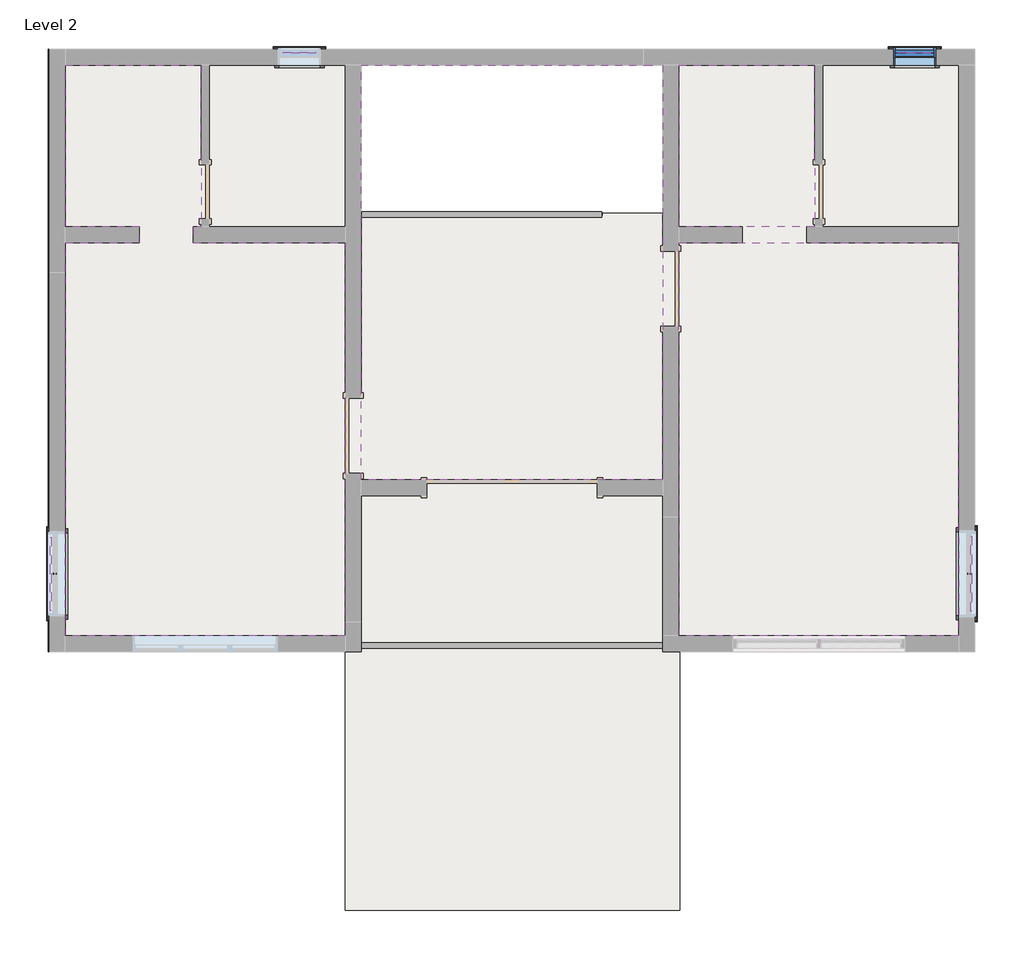
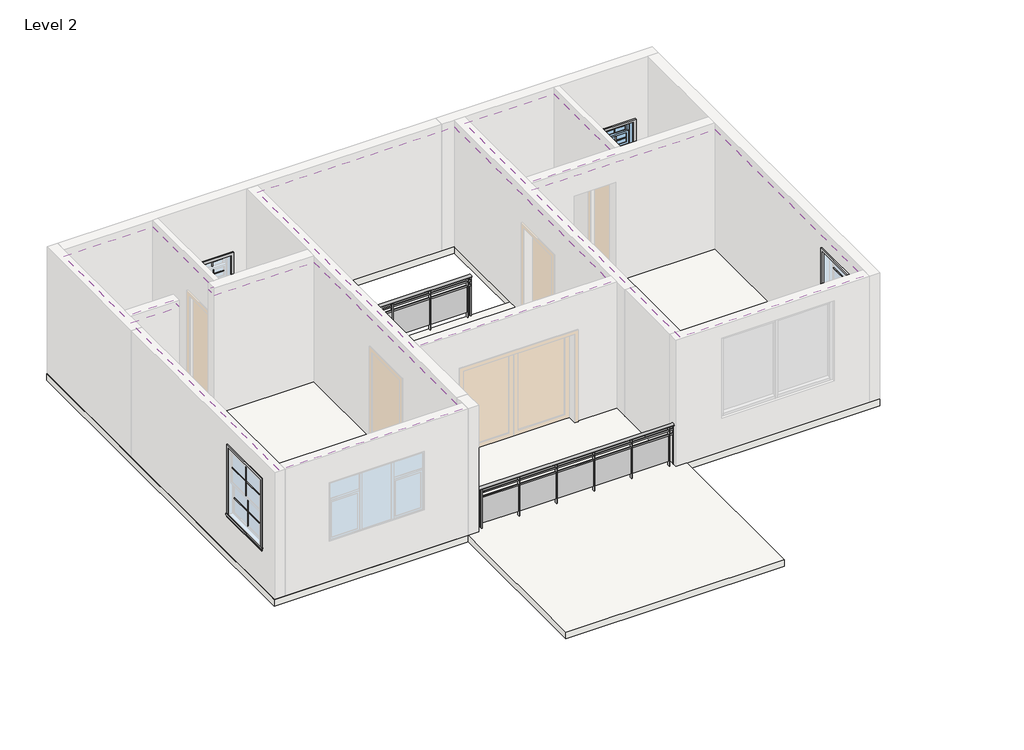
# One storey, part 2 of 2: 16 proxies, 4 coverings, 2 railings, 1 slab, 1 window.
"""IFC4 building model written with IfcOpenShell, lengths in millimetres."""

from ifc_helpers import new_model, si_unit, point, frame, origin, place, context, project, spatial, polyline, ellipse_curve, trimmed, outline, extrude, transform, mapped, element, save
from ifc_brep_helpers import plane_surface, extruded_surface, advanced_brep
from components import muntin_pattern_2x2_muntin_pattern_2x2_872d1288, muntin_pattern_2x2_muntin_pattern_2x2_cfeb24ad, muntin_pattern_2x2_muntin_pattern_2x2_afeb4eca, trim_window_exterior_flat_with_sill_c3105ee7, trim_window_exterior_flat_with_sill_858dc10d, trim_window_exterior_flat_with_sill_92b9b949, trim_window_interior_flat_picture_frame_d5efd988, trim_window_interior_flat_picture_frame_3927330c, trim_window_interior_flat_picture_frame_3bb882cf, window_double_hung_2_x2_15b2d83c

model = new_model("IFC4")

# Units and contexts
model_context = context("Model", 3, world=origin())
ifc_project = project(units=[si_unit("LENGTHUNIT", "METRE", prefix="MILLI")], contexts=[model_context])

# Site, building, storey
site = spatial("IfcSite", under=ifc_project)
building = spatial("IfcBuilding", under=site)
storey = spatial("IfcBuildingStorey", under=building, Name="Level 2", Elevation=3048.0)

# Proxies
placement = place(None, origin())
muntin_pattern_2x2_muntin_pattern_2x2_shape = muntin_pattern_2x2_muntin_pattern_2x2_872d1288(model_context)
element("IfcBuildingElementProxy", 1, Name="Muntin Pattern_2x2 : Muntin Pattern_2x2", ObjectType="Muntin Pattern_2x2 : Muntin Pattern_2x2", at=placement, inside=storey, context=model_context, shape_type="MappedRepresentation", body=[
    mapped(muntin_pattern_2x2_muntin_pattern_2x2_shape, transform((-19390.8072207, 4603.0962903, 4746.625), x_axis=(0.0, 1.0, 0.0), y_axis=(-1.0, 0.0, 0.0), z_axis=(0.0, 0.0, 1.0))),
])
element("IfcBuildingElementProxy", 2, Name="Muntin Pattern_2x2 : Muntin Pattern_2x2", ObjectType="Muntin Pattern_2x2 : Muntin Pattern_2x2", at=placement, inside=storey, context=model_context, shape_type="MappedRepresentation", body=[
    mapped(muntin_pattern_2x2_muntin_pattern_2x2_shape, transform((-19346.3572207, 4603.0962903, 4038.6), x_axis=(0.0, 1.0, 0.0), y_axis=(-1.0, 0.0, 0.0), z_axis=(0.0, 0.0, 1.0))),
])
muntin_pattern_2x2_muntin_pattern_2x2_2_shape = muntin_pattern_2x2_muntin_pattern_2x2_cfeb24ad(model_context)
element("IfcBuildingElementProxy", 3, Name="Muntin Pattern_2x2 : Muntin Pattern_2x2", ObjectType="Muntin Pattern_2x2 : Muntin Pattern_2x2", at=placement, inside=storey, context=model_context, shape_type="MappedRepresentation", body=[
    mapped(muntin_pattern_2x2_muntin_pattern_2x2_2_shape, transform((-15881.0556236, 11998.6707578, 4289.425), x_axis=(1.0, 0.0, 0.0), y_axis=(0.0, 1.0, 0.0), z_axis=(0.0, 0.0, 1.0))),
])
element("IfcBuildingElementProxy", 4, Name="Muntin Pattern_2x2 : Muntin Pattern_2x2", ObjectType="Muntin Pattern_2x2 : Muntin Pattern_2x2", at=placement, inside=storey, context=model_context, shape_type="MappedRepresentation", body=[
    mapped(muntin_pattern_2x2_muntin_pattern_2x2_2_shape, transform((-15881.0556236, 11954.2207578, 4038.6), x_axis=(1.0, 0.0, 0.0), y_axis=(0.0, 1.0, 0.0), z_axis=(0.0, 0.0, 1.0))),
])
element("IfcBuildingElementProxy", 5, Name="Muntin Pattern_2x2 : Muntin Pattern_2x2", ObjectType="Muntin Pattern_2x2 : Muntin Pattern_2x2", at=placement, inside=storey, context=model_context, shape_type="MappedRepresentation", body=[
    mapped(muntin_pattern_2x2_muntin_pattern_2x2_2_shape, transform((-7166.2817031, 11998.6707578, 4289.425), x_axis=(1.0, 0.0, 0.0), y_axis=(0.0, 1.0, 0.0), z_axis=(0.0, 0.0, 1.0))),
])
element("IfcBuildingElementProxy", 6, Name="Muntin Pattern_2x2 : Muntin Pattern_2x2", ObjectType="Muntin Pattern_2x2 : Muntin Pattern_2x2", at=placement, inside=storey, context=model_context, shape_type="MappedRepresentation", body=[
    mapped(muntin_pattern_2x2_muntin_pattern_2x2_2_shape, transform((-7166.2817031, 11954.2207578, 4038.6), x_axis=(1.0, 0.0, 0.0), y_axis=(0.0, 1.0, 0.0), z_axis=(0.0, 0.0, 1.0))),
])
muntin_pattern_2x2_muntin_pattern_2x2_3_shape = muntin_pattern_2x2_muntin_pattern_2x2_afeb4eca(model_context)
element("IfcBuildingElementProxy", 7, Name="Muntin Pattern_2x2 : Muntin Pattern_2x2", ObjectType="Muntin Pattern_2x2 : Muntin Pattern_2x2", at=placement, inside=storey, context=model_context, shape_type="MappedRepresentation", body=[
    mapped(muntin_pattern_2x2_muntin_pattern_2x2_3_shape, transform((-6350.3067031, 4603.0962903, 4746.625), x_axis=(0.0, -1.0, 0.0), y_axis=(1.0, 0.0, 0.0), z_axis=(0.0, 0.0, 1.0))),
])
element("IfcBuildingElementProxy", 8, Name="Muntin Pattern_2x2 : Muntin Pattern_2x2", ObjectType="Muntin Pattern_2x2 : Muntin Pattern_2x2", at=placement, inside=storey, context=model_context, shape_type="MappedRepresentation", body=[
    mapped(muntin_pattern_2x2_muntin_pattern_2x2_3_shape, transform((-6394.7567031, 4603.0962903, 4038.6), x_axis=(0.0, -1.0, 0.0), y_axis=(1.0, 0.0, 0.0), z_axis=(0.0, 0.0, 1.0))),
])
trim_window_exterior_flat_with_sill_shape = trim_window_exterior_flat_with_sill_c3105ee7(model_context)
element("IfcBuildingElementProxy", 9, Name="Trim-Window-Exterior-Flat : with Sill", ObjectType="Trim-Window-Exterior-Flat : with Sill", at=placement, inside=storey, context=model_context, shape_type="MappedRepresentation", body=[
    mapped(trim_window_exterior_flat_with_sill_shape, transform((-19425.7322207, 4603.0962903, 5486.4), x_axis=(0.0, -1.0, 0.0), y_axis=(0.0, 0.0, 1.0), z_axis=(-1.0, 0.0, 0.0))),
])
trim_window_exterior_flat_with_sill_2_shape = trim_window_exterior_flat_with_sill_858dc10d(model_context)
element("IfcBuildingElementProxy", 10, Name="Trim-Window-Exterior-Flat : with Sill", ObjectType="Trim-Window-Exterior-Flat : with Sill", at=placement, inside=storey, context=model_context, shape_type="MappedRepresentation", body=[
    mapped(trim_window_exterior_flat_with_sill_2_shape, transform((-15881.0556236, 12033.5957578, 4572.0), x_axis=(-1.0, 0.0, 0.0), y_axis=(0.0, 0.0, 1.0), z_axis=(0.0, 1.0, 0.0))),
])
element("IfcBuildingElementProxy", 11, Name="Trim-Window-Exterior-Flat : with Sill", ObjectType="Trim-Window-Exterior-Flat : with Sill", at=placement, inside=storey, context=model_context, shape_type="MappedRepresentation", body=[
    mapped(trim_window_exterior_flat_with_sill_2_shape, transform((-7166.2817031, 12033.5957578, 4572.0), x_axis=(-1.0, 0.0, 0.0), y_axis=(0.0, 0.0, 1.0), z_axis=(0.0, 1.0, 0.0))),
])
trim_window_exterior_flat_with_sill_3_shape = trim_window_exterior_flat_with_sill_92b9b949(model_context)
element("IfcBuildingElementProxy", 12, Name="Trim-Window-Exterior-Flat : with Sill", ObjectType="Trim-Window-Exterior-Flat : with Sill", at=placement, inside=storey, context=model_context, shape_type="MappedRepresentation", body=[
    mapped(trim_window_exterior_flat_with_sill_3_shape, transform((-6315.3817031, 4603.0962903, 5486.4), x_axis=(0.0, 1.0, 0.0), y_axis=(0.0, 0.0, 1.0), z_axis=(1.0, 0.0, 0.0))),
])
trim_window_interior_flat_picture_frame_shape = trim_window_interior_flat_picture_frame_d5efd988(model_context)
element("IfcBuildingElementProxy", 13, Name="Trim-Window-Interior-Flat : Picture Frame", ObjectType="Trim-Window-Interior-Flat : Picture Frame", at=placement, inside=storey, context=model_context, shape_type="MappedRepresentation", body=[
    mapped(trim_window_interior_flat_picture_frame_shape, transform((-19197.1322207, 4603.0962903, 5486.4), x_axis=(0.0, 1.0, 0.0), y_axis=(0.0, 0.0, 1.0), z_axis=(1.0, 0.0, 0.0))),
])
trim_window_interior_flat_picture_frame_2_shape = trim_window_interior_flat_picture_frame_3927330c(model_context)
element("IfcBuildingElementProxy", 14, Name="Trim-Window-Interior-Flat : Picture Frame", ObjectType="Trim-Window-Interior-Flat : Picture Frame", at=placement, inside=storey, context=model_context, shape_type="MappedRepresentation", body=[
    mapped(trim_window_interior_flat_picture_frame_2_shape, transform((-15881.0556236, 11804.9957578, 4572.0), x_axis=(1.0, 0.0, 0.0), y_axis=(0.0, 0.0, 1.0), z_axis=(0.0, -1.0, 0.0))),
])
element("IfcBuildingElementProxy", 15, Name="Trim-Window-Interior-Flat : Picture Frame", ObjectType="Trim-Window-Interior-Flat : Picture Frame", at=placement, inside=storey, context=model_context, shape_type="MappedRepresentation", body=[
    mapped(trim_window_interior_flat_picture_frame_2_shape, transform((-7166.2817031, 11804.9957578, 4572.0), x_axis=(1.0, 0.0, 0.0), y_axis=(0.0, 0.0, 1.0), z_axis=(0.0, -1.0, 0.0))),
])
trim_window_interior_flat_picture_frame_3_shape = trim_window_interior_flat_picture_frame_3bb882cf(model_context)
element("IfcBuildingElementProxy", 16, Name="Trim-Window-Interior-Flat : Picture Frame", ObjectType="Trim-Window-Interior-Flat : Picture Frame", at=placement, inside=storey, context=model_context, shape_type="MappedRepresentation", body=[
    mapped(trim_window_interior_flat_picture_frame_3_shape, transform((-6543.9817031, 4603.0962903, 5486.4), x_axis=(0.0, -1.0, 0.0), y_axis=(0.0, 0.0, 1.0), z_axis=(-1.0, 0.0, 0.0))),
])

# Coverings
element("IfcCovering", 17, ObjectType="2' x 4' ACT System", at=placement, inside=storey, context=model_context, shape_type="SweptSolid", body=[
    extrude(outline(polyline([(-6543.9817031, 9289.635577), (-6543.9817031, 3726.7962903), (-10507.7583002, 3726.7962903), (-10507.7583002, 5401.1206207), (-10509.1026022, 5401.1206207), (-10509.1026022, 9289.635577), (-6543.9817031, 9289.635577)])), frame((0.0, 0.0, 5791.2), z_axis=(0.0, 0.0, 1.0), x_axis=(1.0, 0.0, 0.0)), (0.0, 0.0, 1.0), 57.15),
])
element("IfcCovering", 18, ObjectType="2' x 4' ACT System", at=placement, inside=storey, context=model_context, shape_type="SweptSolid", body=[
    extrude(outline(polyline([(-10509.1026022, 9518.235577), (-10509.1026022, 11804.9957578), (-8581.223198, 11804.9957578), (-8581.223198, 9518.235577), (-10509.1026022, 9518.235577)])), frame((0.0, 0.0, 5791.2), z_axis=(0.0, 0.0, 1.0), x_axis=(1.0, 0.0, 0.0)), (0.0, 0.0, 1.0), 57.15),
])
element("IfcCovering", 19, ObjectType="2' x 4' ACT System", at=placement, inside=storey, context=model_context, shape_type="SweptSolid", body=[
    extrude(outline(polyline([(-15004.7556236, 5935.1163046), (-15004.7556236, 11804.9957578), (-11009.5531945, 11804.9957578), (-10737.7026022, 11804.9957578), (-10737.7026022, 5935.1163046), (-15004.7556236, 5935.1163046)])), frame((0.0, 0.0, 5791.2), z_axis=(0.0, 0.0, 1.0), x_axis=(1.0, 0.0, 0.0)), (0.0, 0.0, 1.0), 57.15),
])
element("IfcCovering", 20, ObjectType="2' x 4' ACT System", at=placement, inside=storey, context=model_context, shape_type="SweptSolid", body=[
    extrude(outline(polyline([(-19197.1322207, 9290.2207935), (-18149.1852461, 9290.2207935), (-18149.1852461, 9518.8207935), (-19197.1322207, 9518.8207935), (-19197.1322207, 11804.9957578), (-17272.3740665, 11804.9957578), (-17272.3740665, 9518.8207935), (-17388.0183685, 9518.8207935), (-17388.0183685, 9290.2207935), (-15233.3556236, 9290.2207935), (-15233.3556236, 3726.7962903), (-19197.1322207, 3726.7962903), (-19197.1322207, 9290.2207935)])), frame((0.0, 0.0, 5791.2), z_axis=(0.0, 0.0, 1.0), x_axis=(1.0, 0.0, 0.0)), (0.0, 0.0, 1.0), 57.15),
])

# Railings
element("IfcRailing", 21, ObjectType="Glass Panel - Bottom Fill", at=placement, inside=storey, context=model_context, shape_type="SolidModel", body=[
    advanced_brep(
    [(-15004.5982861, 9732.8204925, 3962.4), (-15004.5982861, 9656.6204925, 3962.4), (-11600.9982861, 9732.8204925, 3962.4), (-11600.9982861, 9656.6204925, 3962.4)],
    [
        (0, 1, ellipse_curve(frame((-15004.5982861, 9694.7204925, 3962.4), z_axis=(-1.0, 0.0, 0.0), x_axis=(0.0, -1.0, 0.0)), 38.1, 28.575)),
        (1, 0, ellipse_curve(frame((-15004.5982861, 9694.7204925, 3962.4), z_axis=(-1.0, 0.0, 0.0), x_axis=(0.0, -1.0, 0.0)), 38.1, 28.575)),
        (2, 3, ellipse_curve(frame((-11600.9982861, 9694.7204925, 3962.4), z_axis=(1.0, 0.0, 0.0), x_axis=(0.0, -1.0, 0.0)), 38.1, 28.575)),
        (3, 2, ellipse_curve(frame((-11600.9982861, 9694.7204925, 3962.4), z_axis=(1.0, 0.0, 0.0), x_axis=(0.0, -1.0, 0.0)), 38.1, 28.575)),
        (0, 2),
        (3, 1),
    ],
    [
        plane_surface(frame((-15004.5982861, 9694.7204925, 3962.4), z_axis=(-1.0, 0.0, 0.0), x_axis=(0.0, 1.0, 0.0))),
        plane_surface(frame((-11600.9982861, 9694.7204925, 3962.4), z_axis=(1.0, 0.0, 0.0), x_axis=(0.0, 1.0, 0.0))),
        extruded_surface(trimmed(ellipse_curve(frame((-11600.9982861, 9694.7204925, 3962.4), z_axis=(-1.0, 0.0, 0.0), x_axis=(0.0, -1.0, 0.0)), 38.1, 28.575), [point((-11600.9982861, 9732.8204925, 3962.4))], [point((-11600.9982861, 9656.6204925, 3962.4))], True, "CARTESIAN"), (-3403.5999999999985, 0.0, 0.0), 3403.5999999999985),
        extruded_surface(trimmed(ellipse_curve(frame((-11600.9982861, 9694.7204925, 3962.4), z_axis=(-1.0, 0.0, 0.0), x_axis=(0.0, -1.0, 0.0)), 38.1, 28.575), [point((-11600.9982861, 9656.6204925, 3962.4))], [point((-11600.9982861, 9732.8204925, 3962.4))], True, "CARTESIAN"), (-3403.5999999999985, 0.0, 0.0), 3403.5999999999985),
    ],
    [
        (0, [[1, 2]]),
        (1, [[3, 4]]),
        (2, [[-1, 5, -4, 6]]),
        (3, [[-2, -6, -3, -5]]),
    ],
),
    extrude(outline(polyline([(-15004.5982861, 9682.0204925), (-15004.5982861, 9707.4204925), (-11600.9982861, 9707.4204925), (-11600.9982861, 9682.0204925), (-15004.5982861, 9682.0204925)])), frame((0.0, 0.0, 3848.1), z_axis=(0.0, 0.0, 1.0), x_axis=(1.0, 0.0, 0.0)), (0.0, 0.0, 1.0), 25.4),
    extrude(outline(polyline([(-15004.5982861, 9682.0204925), (-15004.5982861, 9707.4204925), (-11600.9982861, 9707.4204925), (-11600.9982861, 9682.0204925), (-15004.5982861, 9682.0204925)])), frame((0.0, 0.0, 3746.5), z_axis=(0.0, 0.0, 1.0), x_axis=(1.0, 0.0, 0.0)), (0.0, 0.0, 1.0), 25.4),
    extrude(outline(polyline([(-11683.5482861, 9669.3204925), (-11683.5482861, 9720.1204925), (-11670.8482861, 9720.1204925), (-11670.8482861, 9669.3204925), (-11683.5482861, 9669.3204925)])), frame((0.0, 0.0, 3048.0), z_axis=(0.0, 0.0, 1.0), x_axis=(1.0, 0.0, 0.0)), (0.0, 0.0, 1.0), 885.825),
    extrude(outline(polyline([(-12489.9982861, 9701.2556495), (-11677.1982861, 9701.2556495), (-11677.1982861, 9694.9056495), (-12489.9982861, 9694.9056495), (-12489.9982861, 9701.2556495)])), frame((0.0, 0.0, 3149.6), z_axis=(0.0, 0.0, 1.0), x_axis=(1.0, 0.0, 0.0)), (0.0, 0.0, 1.0), 596.9),
    extrude(outline(polyline([(-12496.3482861, 9669.3204925), (-12496.3482861, 9720.1204925), (-12483.6482861, 9720.1204925), (-12483.6482861, 9669.3204925), (-12496.3482861, 9669.3204925)])), frame((0.0, 0.0, 3048.0), z_axis=(0.0, 0.0, 1.0), x_axis=(1.0, 0.0, 0.0)), (0.0, 0.0, 1.0), 885.825),
    extrude(outline(polyline([(-13302.7982861, 9701.2556495), (-12489.9982861, 9701.2556495), (-12489.9982861, 9694.9056495), (-13302.7982861, 9694.9056495), (-13302.7982861, 9701.2556495)])), frame((0.0, 0.0, 3149.6), z_axis=(0.0, 0.0, 1.0), x_axis=(1.0, 0.0, 0.0)), (0.0, 0.0, 1.0), 596.9),
    extrude(outline(polyline([(-13309.1482861, 9669.3204925), (-13309.1482861, 9720.1204925), (-13296.4482861, 9720.1204925), (-13296.4482861, 9669.3204925), (-13309.1482861, 9669.3204925)])), frame((0.0, 0.0, 3048.0), z_axis=(0.0, 0.0, 1.0), x_axis=(1.0, 0.0, 0.0)), (0.0, 0.0, 1.0), 885.825),
    extrude(outline(polyline([(-14115.5982861, 9701.2556495), (-13302.7982861, 9701.2556495), (-13302.7982861, 9694.9056495), (-14115.5982861, 9694.9056495), (-14115.5982861, 9701.2556495)])), frame((0.0, 0.0, 3149.6), z_axis=(0.0, 0.0, 1.0), x_axis=(1.0, 0.0, 0.0)), (0.0, 0.0, 1.0), 596.9),
    extrude(outline(polyline([(-14121.9482861, 9669.3204925), (-14121.9482861, 9720.1204925), (-14109.2482861, 9720.1204925), (-14109.2482861, 9669.3204925), (-14121.9482861, 9669.3204925)])), frame((0.0, 0.0, 3048.0), z_axis=(0.0, 0.0, 1.0), x_axis=(1.0, 0.0, 0.0)), (0.0, 0.0, 1.0), 885.825),
    extrude(outline(polyline([(-14928.3982861, 9701.2556495), (-14115.5982861, 9701.2556495), (-14115.5982861, 9694.9056495), (-14928.3982861, 9694.9056495), (-14928.3982861, 9701.2556495)])), frame((0.0, 0.0, 3149.6), z_axis=(0.0, 0.0, 1.0), x_axis=(1.0, 0.0, 0.0)), (0.0, 0.0, 1.0), 596.9),
    extrude(outline(polyline([(-14934.7482861, 9669.3204925), (-14934.7482861, 9720.1204925), (-14922.0482861, 9720.1204925), (-14922.0482861, 9669.3204925), (-14934.7482861, 9669.3204925)])), frame((0.0, 0.0, 3048.0), z_axis=(0.0, 0.0, 1.0), x_axis=(1.0, 0.0, 0.0)), (0.0, 0.0, 1.0), 885.825),
    extrude(outline(polyline([(-11613.6982861, 9685.1954925), (-11613.6982861, 9704.2454925), (-11594.6482861, 9704.2454925), (-11594.6482861, 9685.1954925), (-11613.6982861, 9685.1954925)])), frame((0.0, 0.0, 3048.0), z_axis=(0.0, 0.0, 1.0), x_axis=(1.0, 0.0, 0.0)), (0.0, 0.0, 1.0), 885.825),
    extrude(outline(polyline([(-15010.9482861, 9685.1954925), (-15010.9482861, 9704.2454925), (-14991.8982861, 9704.2454925), (-14991.8982861, 9685.1954925), (-15010.9482861, 9685.1954925)])), frame((0.0, 0.0, 3048.0), z_axis=(0.0, 0.0, 1.0), x_axis=(1.0, 0.0, 0.0)), (0.0, 0.0, 1.0), 885.825),
])
element("IfcRailing", 22, ObjectType="Glass Panel - Bottom Fill", at=placement, inside=storey, context=model_context, shape_type="SolidModel", body=[
    advanced_brep(
    [(-15004.5982861, 3624.2466339, 3962.4), (-15004.5982861, 3548.0466339, 3962.4), (-10733.9149392, 3624.2466339, 3962.4), (-10733.9149392, 3548.0466339, 3962.4)],
    [
        (0, 1, ellipse_curve(frame((-15004.5982861, 3586.1466339, 3962.4), z_axis=(-1.0, 0.0, 0.0), x_axis=(0.0, -1.0, 0.0)), 38.1, 28.575)),
        (1, 0, ellipse_curve(frame((-15004.5982861, 3586.1466339, 3962.4), z_axis=(-1.0, 0.0, 0.0), x_axis=(0.0, -1.0, 0.0)), 38.1, 28.575)),
        (2, 3, ellipse_curve(frame((-10733.9149392, 3586.1466339, 3962.4), z_axis=(1.0, 0.0, 0.0), x_axis=(0.0, -1.0, 0.0)), 38.1, 28.575)),
        (3, 2, ellipse_curve(frame((-10733.9149392, 3586.1466339, 3962.4), z_axis=(1.0, 0.0, 0.0), x_axis=(0.0, -1.0, 0.0)), 38.1, 28.575)),
        (0, 2),
        (3, 1),
    ],
    [
        plane_surface(frame((-15004.5982861, 3586.1466339, 3962.4), z_axis=(-1.0, 0.0, 0.0), x_axis=(0.0, 1.0, 0.0))),
        plane_surface(frame((-10733.9149392, 3586.1466339, 3962.4), z_axis=(1.0, 0.0, 0.0), x_axis=(0.0, 1.0, 0.0))),
        extruded_surface(trimmed(ellipse_curve(frame((-10733.9149392, 3586.1466339, 3962.4), z_axis=(-1.0, 0.0, 0.0), x_axis=(0.0, -1.0, 0.0)), 38.1, 28.575), [point((-10733.9149392, 3624.2466339, 3962.4))], [point((-10733.9149392, 3548.0466339, 3962.4))], True, "CARTESIAN"), (-4270.683346899999, 0.0, 0.0), 4270.683346899999),
        extruded_surface(trimmed(ellipse_curve(frame((-10733.9149392, 3586.1466339, 3962.4), z_axis=(-1.0, 0.0, 0.0), x_axis=(0.0, -1.0, 0.0)), 38.1, 28.575), [point((-10733.9149392, 3548.0466339, 3962.4))], [point((-10733.9149392, 3624.2466339, 3962.4))], True, "CARTESIAN"), (-4270.683346899999, 0.0, 0.0), 4270.683346899999),
    ],
    [
        (0, [[1, 2]]),
        (1, [[3, 4]]),
        (2, [[-1, 5, -4, 6]]),
        (3, [[-2, -6, -3, -5]]),
    ],
),
    extrude(outline(polyline([(-15004.5982861, 3573.4466339), (-15004.5982861, 3598.8466339), (-10733.9149392, 3598.8466339), (-10733.9149392, 3573.4466339), (-15004.5982861, 3573.4466339)])), frame((0.0, 0.0, 3848.1), z_axis=(0.0, 0.0, 1.0), x_axis=(1.0, 0.0, 0.0)), (0.0, 0.0, 1.0), 25.4),
    extrude(outline(polyline([(-15004.5982861, 3573.4466339), (-15004.5982861, 3598.8466339), (-10733.9149392, 3598.8466339), (-10733.9149392, 3573.4466339), (-15004.5982861, 3573.4466339)])), frame((0.0, 0.0, 3746.5), z_axis=(0.0, 0.0, 1.0), x_axis=(1.0, 0.0, 0.0)), (0.0, 0.0, 1.0), 25.4),
    extrude(outline(polyline([(-10843.6066127, 3560.7466339), (-10843.6066127, 3611.5466339), (-10830.9066127, 3611.5466339), (-10830.9066127, 3560.7466339), (-10843.6066127, 3560.7466339)])), frame((0.0, 0.0, 3048.0), z_axis=(0.0, 0.0, 1.0), x_axis=(1.0, 0.0, 0.0)), (0.0, 0.0, 1.0), 885.825),
    extrude(outline(polyline([(-11650.0566127, 3592.6817909), (-10837.2566127, 3592.6817909), (-10837.2566127, 3586.3317909), (-11650.0566127, 3586.3317909), (-11650.0566127, 3592.6817909)])), frame((0.0, 0.0, 3149.6), z_axis=(0.0, 0.0, 1.0), x_axis=(1.0, 0.0, 0.0)), (0.0, 0.0, 1.0), 596.9),
    extrude(outline(polyline([(-11656.4066127, 3560.7466339), (-11656.4066127, 3611.5466339), (-11643.7066127, 3611.5466339), (-11643.7066127, 3560.7466339), (-11656.4066127, 3560.7466339)])), frame((0.0, 0.0, 3048.0), z_axis=(0.0, 0.0, 1.0), x_axis=(1.0, 0.0, 0.0)), (0.0, 0.0, 1.0), 885.825),
    extrude(outline(polyline([(-12462.8566127, 3592.6817909), (-11650.0566127, 3592.6817909), (-11650.0566127, 3586.3317909), (-12462.8566127, 3586.3317909), (-12462.8566127, 3592.6817909)])), frame((0.0, 0.0, 3149.6), z_axis=(0.0, 0.0, 1.0), x_axis=(1.0, 0.0, 0.0)), (0.0, 0.0, 1.0), 596.9),
    extrude(outline(polyline([(-12469.2066127, 3560.7466339), (-12469.2066127, 3611.5466339), (-12456.5066127, 3611.5466339), (-12456.5066127, 3560.7466339), (-12469.2066127, 3560.7466339)])), frame((0.0, 0.0, 3048.0), z_axis=(0.0, 0.0, 1.0), x_axis=(1.0, 0.0, 0.0)), (0.0, 0.0, 1.0), 885.825),
    extrude(outline(polyline([(-13275.6566127, 3592.6817909), (-12462.8566127, 3592.6817909), (-12462.8566127, 3586.3317909), (-13275.6566127, 3586.3317909), (-13275.6566127, 3592.6817909)])), frame((0.0, 0.0, 3149.6), z_axis=(0.0, 0.0, 1.0), x_axis=(1.0, 0.0, 0.0)), (0.0, 0.0, 1.0), 596.9),
    extrude(outline(polyline([(-13282.0066127, 3560.7466339), (-13282.0066127, 3611.5466339), (-13269.3066127, 3611.5466339), (-13269.3066127, 3560.7466339), (-13282.0066127, 3560.7466339)])), frame((0.0, 0.0, 3048.0), z_axis=(0.0, 0.0, 1.0), x_axis=(1.0, 0.0, 0.0)), (0.0, 0.0, 1.0), 885.825),
    extrude(outline(polyline([(-14088.4566127, 3592.6817909), (-13275.6566127, 3592.6817909), (-13275.6566127, 3586.3317909), (-14088.4566127, 3586.3317909), (-14088.4566127, 3592.6817909)])), frame((0.0, 0.0, 3149.6), z_axis=(0.0, 0.0, 1.0), x_axis=(1.0, 0.0, 0.0)), (0.0, 0.0, 1.0), 596.9),
    extrude(outline(polyline([(-14094.8066127, 3560.7466339), (-14094.8066127, 3611.5466339), (-14082.1066127, 3611.5466339), (-14082.1066127, 3560.7466339), (-14094.8066127, 3560.7466339)])), frame((0.0, 0.0, 3048.0), z_axis=(0.0, 0.0, 1.0), x_axis=(1.0, 0.0, 0.0)), (0.0, 0.0, 1.0), 885.825),
    extrude(outline(polyline([(-14901.2566127, 3592.6817909), (-14088.4566127, 3592.6817909), (-14088.4566127, 3586.3317909), (-14901.2566127, 3586.3317909), (-14901.2566127, 3592.6817909)])), frame((0.0, 0.0, 3149.6), z_axis=(0.0, 0.0, 1.0), x_axis=(1.0, 0.0, 0.0)), (0.0, 0.0, 1.0), 596.9),
    extrude(outline(polyline([(-14907.6066127, 3560.7466339), (-14907.6066127, 3611.5466339), (-14894.9066127, 3611.5466339), (-14894.9066127, 3560.7466339), (-14907.6066127, 3560.7466339)])), frame((0.0, 0.0, 3048.0), z_axis=(0.0, 0.0, 1.0), x_axis=(1.0, 0.0, 0.0)), (0.0, 0.0, 1.0), 885.825),
    extrude(outline(polyline([(-10746.6149392, 3576.6216339), (-10746.6149392, 3595.6716339), (-10727.5649392, 3595.6716339), (-10727.5649392, 3576.6216339), (-10746.6149392, 3576.6216339)])), frame((0.0, 0.0, 3048.0), z_axis=(0.0, 0.0, 1.0), x_axis=(1.0, 0.0, 0.0)), (0.0, 0.0, 1.0), 885.825),
    extrude(outline(polyline([(-15010.9482861, 3576.6216339), (-15010.9482861, 3595.6716339), (-14991.8982861, 3595.6716339), (-14991.8982861, 3576.6216339), (-15010.9482861, 3576.6216339)])), frame((0.0, 0.0, 3048.0), z_axis=(0.0, 0.0, 1.0), x_axis=(1.0, 0.0, 0.0)), (0.0, 0.0, 1.0), 885.825),
])

# Slab
element("IfcSlab", 23, ObjectType="6\"", at=placement, inside=storey, context=model_context, shape_type="SweptSolid", body=[
    extrude(outline(polyline([(-6312.7810046, 12034.9129661), (-6312.7810046, 3498.1962903), (-10495.4973413, 3498.1962903), (-10495.4973413, -161.4013365), (-15231.4325054, -161.4013365), (-15231.4325054, 3498.1962903), (-19437.2989325, 3498.1962903), (-19437.2989325, 12034.9129661), (-6312.7810046, 12034.9129661)]), holes=[polyline([(-10733.9149392, 11803.4453953), (-15004.5982861, 11803.4453953), (-15004.5982861, 9720.1872586), (-10733.9149392, 9720.1872586), (-10733.9149392, 11803.4453953)])]), frame((0.0, 0.0, 2895.6), z_axis=(0.0, 0.0, 1.0), x_axis=(1.0, 0.0, 0.0)), (0.0, 0.0, 1.0), 152.4),
])

# Window
window_double_hung_2_x2_shape = window_double_hung_2_x2_15b2d83c(model_context)
element("IfcWindow", 24, ObjectType="Window-Double-Hung : 2'x2'", at=placement, inside=storey, context=model_context, shape_type="MappedRepresentation", body=[
    mapped(window_double_hung_2_x2_shape, transform((-7166.2817031, 11919.2957578, 3048.0), x_axis=(1.0, 0.0, 0.0), y_axis=(0.0, 1.0, 0.0), z_axis=(0.0, 0.0, 1.0))),
])

save(model, "model.ifc")

# Revit data of these elements
# Type "Muntin Pattern_2x2 : Muntin Pattern_2x2"
#   Width [instance default] = 4' - 0"
#   Thickness = 0' - 0 1/2"
#   Height [instance default] = 4' - 0"
#   Distance = 0' - 0 3/4"
#   Interior Material [instance default] = none
#   Exterior Material [instance default] = none
#   Default Elevation = 0
# Type "Trim-Window-Exterior-Flat : with Sill"
#   Trim Width = 0' - 2 1/4"
#   Trim Thickness_Picture Frame = 0' - 1 1/4"
#   Trim Thickness_with Sill = 0' - 0 3/4"
#   Sill Thickness = 0' - 1 1/4"
#   Opening Width [instance default] = 2' - 0"
#   Opening Height [instance default] = 3' - 0"
#   Default Elevation = 4' - 0"
#   Sill = yes
#   Picture Frame = no
#   Trim Material [instance default] = none
# Type "Trim-Window-Interior-Flat : Picture Frame"
#   Trim Thickness_Picture Frame = 0' - 1 1/4"
#   Trim Width = 0' - 2 1/4"
#   Trim Thickness_with Sill = 0' - 0 3/4"
#   Sill Thickness = 0' - 1 1/4"
#   Opening Width [instance default] = 2' - 0"
#   Opening Height [instance default] = 3' - 0"
#   Default Elevation = 4' - 0"
#   Sill = no
#   Picture Frame = yes
#   Trim Material [instance default] = none
# Type "2' x 4' ACT System"
#   Assembly Code = "C3030210"
#   built-in parameter 1002203 = 1 (stored number, unit not read)
#   built-in parameter 1002202 = 1 (stored number, unit not read)
#   Layers, outside or top first: 0' - 1 5/8" "Default" (function 1); 0' - 0 5/8" "Acoustic Ceiling Tile 24 x 48" (function 5)
# Type "Glass Panel - Bottom Fill"
#   Assembly Code = "C2010400"
#   built-in parameter 1008612 = 0.0416667 (stored number, unit not read)
#   built-in parameter 1008611 = 0.0416667 (stored number, unit not read)
#   built-in parameter 1008609 = 0.333333 (stored number, unit not read)
#   built-in parameter 1008604 = 0.166667 (stored number, unit not read)
#   built-in parameter 1008603 = 0.166667 (stored number, unit not read)
#   Railing Height = 3' - 0"
#   built-in parameter 1008630 = 2
#   built-in parameter 1008610 = 2
#   built-in parameter 1008618 = Baluster - Square : 3/4"
# Type "6\""
#   Assembly Code = "B1010"
#   Function = 0
#   Layers, outside or top first: 0' - 6" no material (function 1)
# Type "Window-Double-Hung : 2'x2'"
#   Type Mark = "26"
#   Fire Rating = "0.5h"
#   Construction Type Id = "DG-DR"
#   Assembly Code = "B2020100"
#   Analytic Construction = "Double glazing - domestic"
#   Wall Thickness [instance default] = 0' - 6"
#   Window Inset [instance default] = 0' - 0"
#   Visual Light Transmittance = 0.81
#   Thermal Resistance (R) = 1.8146 (h·ft²·°F)/BTU
#   Solar Heat Gain Coefficient = 0.76
#   Muntin Width = 1' - 6"
#   Muntin Height = 0' - 8 1/8"
#   Interior Wall Closure [instance default] = 0' - 1 1/2"
#   Rough Width = 2' - 0 1/2"
#   Rough Height = 2' - 0 1/2"
#   Frame Extension [instance default] = 0' - 1 1/4"
#   Exterior Wall Closure [instance default] = 0' - 0 1/2"
#   Extension Jamb [instance default] = 0' - 1 1/2"
#   Heat Transfer Coefficient (U) = 0.5511 BTU/(h·ft²·°F)
#   Height = 2' - 0"
#   Width = 2' - 0"
#   Top Muntin Visibility = yes
#   Indicator Visibility [instance default] = yes
#   Extension Jamb Visibility [instance default] = yes
#   Interior Trim Visibility [instance default] = yes
#   Exterior Trim Visibility [instance default] = yes
#   Define Thermal Properties by = 1
#   Bottom Muntin Visibility = yes
#   Muntin Pattern = Muntin Pattern_2x2 : Muntin Pattern_2x2
#   Interior Trim Material = Wood - Stained
#   Interior Trim = Trim-Window-Interior-Flat : Picture Frame
#   Exterior Trim Material = Clad - White
#   Exterior Trim = Trim-Window-Exterior-Flat : with Sill
#   Glass Panel Material = Glass
#   Exterior Frame Material = Clad - White
#   Interior Frame Material = Wood - Stained
#   Wall Closure = (empty or 0)
# Elements 1, 2 (IfcBuildingElementProxy, "Muntin Pattern_2x2 : Muntin Pattern_2x2")
#   Width = 3' - 5"
#   Height = 2' - 2 1/8"
#   Interior Material = Wood - Stained
#   Exterior Material = Clad - White
#   Phase Created = New Construction
#   Materials on its faces: "Clad - White", "Wood - Stained"
# Elements 3, 4, 5, 6 (IfcBuildingElementProxy, "Muntin Pattern_2x2 : Muntin Pattern_2x2")
#   Width = 1' - 6"
#   Height = 0' - 8 1/8"
#   Interior Material = Wood - Stained
#   Exterior Material = Clad - White
#   Phase Created = New Construction
#   Materials on its faces: "Clad - White", "Wood - Stained"
# Elements 7, 8 (IfcBuildingElementProxy, "Muntin Pattern_2x2 : Muntin Pattern_2x2")
#   Width = 3' - 6"
#   Height = 2' - 2 1/8"
#   Interior Material = Wood - Stained
#   Exterior Material = Clad - White
#   Phase Created = New Construction
#   Materials on its faces: "Clad - White", "Wood - Stained"
# Element 9 (IfcBuildingElementProxy, "Trim-Window-Exterior-Flat : with Sill")
#   Opening Width = 3' - 11"
#   Opening Height = 5' - 0"
#   Trim Material = Clad - White
#   Phase Created = New Construction
#   Materials on its faces: "Clad - White"
# Elements 10, 11 (IfcBuildingElementProxy, "Trim-Window-Exterior-Flat : with Sill")
#   Opening Width = 2' - 0"
#   Opening Height = 2' - 0"
#   Trim Material = Clad - White
#   Phase Created = New Construction
#   Materials on its faces: "Clad - White"
# Element 12 (IfcBuildingElementProxy, "Trim-Window-Exterior-Flat : with Sill")
#   Opening Width = 4' - 0"
#   Opening Height = 5' - 0"
#   Trim Material = Clad - White
#   Phase Created = New Construction
#   Materials on its faces: "Clad - White"
# Element 13 (IfcBuildingElementProxy, "Trim-Window-Interior-Flat : Picture Frame")
#   Opening Width = 3' - 11"
#   Opening Height = 5' - 0"
#   Trim Material = Wood - Stained
#   Phase Created = New Construction
#   Materials on its faces: "Wood - Stained"
# Elements 14, 15 (IfcBuildingElementProxy, "Trim-Window-Interior-Flat : Picture Frame")
#   Opening Width = 2' - 0"
#   Opening Height = 2' - 0"
#   Trim Material = Wood - Stained
#   Phase Created = New Construction
#   Materials on its faces: "Wood - Stained"
# Element 16 (IfcBuildingElementProxy, "Trim-Window-Interior-Flat : Picture Frame")
#   Opening Width = 4' - 0"
#   Opening Height = 5' - 0"
#   Trim Material = Wood - Stained
#   Phase Created = New Construction
#   Materials on its faces: "Wood - Stained"
# Elements 17, 18, 19, 20 (IfcCovering, "2' x 4' ACT System")
#   Height Offset From Level = 9' - 0"
#   Phase Created = New Construction
#   Materials on its faces: "Acoustic Ceiling Tile 24 x 48", "Default"
# Elements 21, 22 (IfcRailing, "Glass Panel - Bottom Fill")
#   Phase Created = New Construction
#   Materials on its faces: "Glass"
# Element 23 (IfcSlab, "6\"")
#   Height Offset From Level = 0' - 0"
#   Phase Created = New Construction
#   Materials on its faces: "Default Floor"
# Element 24 (IfcWindow, "Window-Double-Hung : 2'x2'")
#   Mark = "13"
#   Window Inset = 0' - 0"
#   Interior Wall Closure = 0' - 1 1/2"
#   Frame Extension = 0' - 1 1/4"
#   Exterior Wall Closure = 0' - 0 1/2"
#   Interior Trim Visibility = yes
#   Indicator Visibility = yes
#   Exterior Trim Visibility = yes
#   Phase Created = New Construction
#   Materials on its faces: "Wood - Stained", "Glass", "Clad - White"
# Materials
#   "Default": colour RGB 127 127 127, transparency 0, Cost = 0
#   "Acoustic Ceiling Tile 24 x 48": class "Generic", colour RGB 229 229 229, transparency 0, Description = "Acoustic Ceiling Tile 24 x 48", Cost = 0
#   "Wood - Stained": class "Wood", colour RGB 224 178 126, transparency 0, Cost = 0
#   "Clad - White": class "Wood", colour RGB 242 242 238, transparency 0, Cost = 0
#   "Glass": class "Glass", colour RGB 154 182 205, transparency 0.85, Description = "Soda Lime Glass", Cost = 0
#   "Default Floor": colour RGB 128 128 128, transparency 0, Cost = 0
